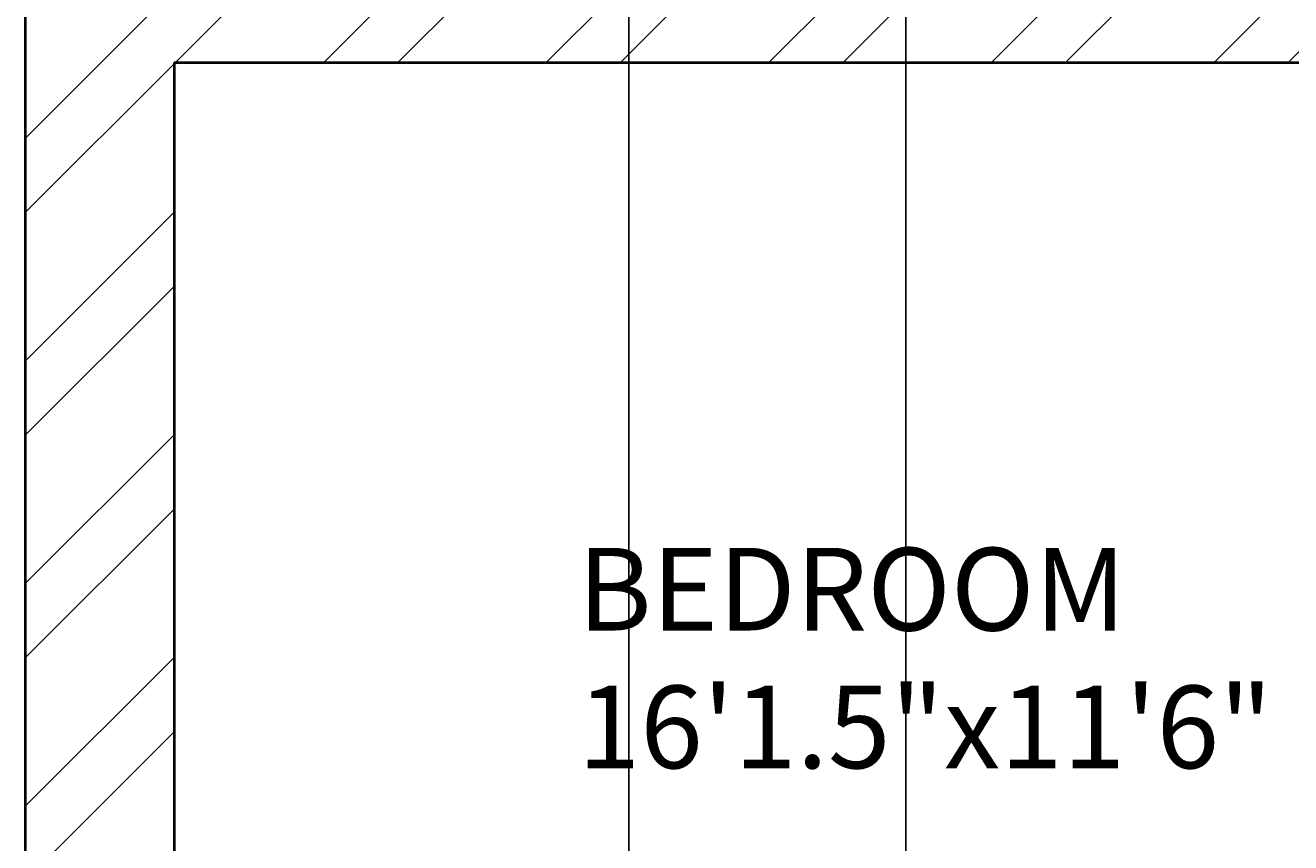
# Model space of a CAD drawing. Units: inches. Extents: x 1601 to 2297, y 1496 to 2631.
# Tile 34 of 57: x 1686 to 1763, y 2236 to 2286. Entities that reach past the tile are written whole.
import ezdxf

# ---------------------------------------------------------------- set-up
doc = ezdxf.new("R2010")
doc.units = ezdxf.units.IN
for name, color, linetype, lineweight in [('A-ANNO-DIMS', 2, 'Continuous', 18), ('A-AREA-IDEN', 7, 'Continuous', 18), ('A-WALL', 7, 'Continuous', 40), ('A-WALL-PATT', 215, 'Continuous', 13)]:
    doc.layers.add(name, color=color, linetype=linetype, lineweight=lineweight)
doc.styles.get("Standard").update_dxf_attribs({"font": 'arial.ttf'})
doc.dimstyles.get("Standard").update_dxf_attribs({"dimtxt": 0.18, "dimasz": 0.18, "dimexe": 0.18, "dimexo": 0.0625, "dimgap": 0.09, "dimtad": 0, "dimtih": 1, "dimtoh": 1, "dimdec": 4, "dimzin": 0, "dimdsep": 46, "dimtxsty": 'Standard', "dimcen": 0.09, "dimadec": 0, "dimazin": 0, "dimtfac": 1, "dimtdec": 4, "dimtofl": 0, "dimtmove": 0, "dimatfit": 3, "dimfxl": 1, "dimtolj": 1, "dimtzin": 0, "dimarcsym": 0})

# ---------------------------------------------------------------- blocks, each defined once
blk = doc.blocks.new('*D32')
at = {"layer": 'A-ANNO-DIMS', "color": 0, "lineweight": -2, "transparency": 16777216}
for p, q in [((1686.037, 2031.388), (1686.037, 2581.055)), ((1686.217, 2580.875), (1703.909, 2580.875)), ((1722.389, 2580.875), (1704.697, 2580.875)), ((1722.569, 2031.388), (1722.569, 2581.055))]:
    blk.add_line(p, q, dxfattribs=at)
at = {"layer": 'A-ANNO-DIMS', "color": 0, "transparency": 16777216}
for points in [[(1686.217, 2580.905), (1686.217, 2580.845), (1686.037, 2580.875)], [(1722.389, 2580.905), (1722.389, 2580.845), (1722.569, 2580.875)]]:
    blk.add_solid(points, dxfattribs=at)
at = {"layer": 'Defpoints', "color": 0, "transparency": 16777216}
for p in [(1722.569, 2580.875), (1686.037, 2031.325), (1722.569, 2031.325)]:
    blk.add_point(p, dxfattribs=at)
at = {"layer": 'A-ANNO-DIMS', "color": 0, "transparency": 16777216, "insert": (1704.303, 2580.875), "char_height": 0.18, "attachment_point": 5}
blk.add_mtext('\\A1;36.53', dxfattribs=at)
blk = doc.blocks.new('*D36')
at = {"layer": 'A-ANNO-DIMS', "color": 0, "lineweight": -2, "transparency": 16777216}
for p, q in [((1686.037, 1635.388), (1686.037, 2581.055)), ((1686.217, 2580.875), (1712.362, 2580.875)), ((1739.154, 2580.875), (1713.009, 2580.875)), ((1739.334, 1635.388), (1739.334, 2581.055))]:
    blk.add_line(p, q, dxfattribs=at)
at = {"layer": 'A-ANNO-DIMS', "color": 0, "transparency": 16777216}
for points in [[(1686.217, 2580.905), (1686.217, 2580.845), (1686.037, 2580.875)], [(1739.154, 2580.905), (1739.154, 2580.845), (1739.334, 2580.875)]]:
    blk.add_solid(points, dxfattribs=at)
at = {"layer": 'Defpoints', "color": 0, "transparency": 16777216}
for p in [(1739.334, 2580.875), (1686.037, 1635.325), (1739.334, 1635.325)]:
    blk.add_point(p, dxfattribs=at)
at = {"layer": 'A-ANNO-DIMS', "color": 0, "transparency": 16777216, "insert": (1712.685, 2580.875), "char_height": 0.18, "attachment_point": 5}
blk.add_mtext('\\A1;53.3', dxfattribs=at)

msp = doc.modelspace()

# ---------------------------------------------------------------- hatches: boundary and pattern name
at = {"layer": 'A-WALL-PATT'}
h = msp.add_hatch(dxfattribs=at)
h.set_pattern_fill('ANSI32', color=256)
h.paths.add_polyline_path([(1842.0336, 2528.0767), (1842.0336, 2532.3254), (1686.0373, 2532.3254), (1686.0373, 2492.9493), (1695.0373, 2492.9493), (1695.0373, 2523.3254), (1827.0373, 2523.3254), (1827.0373, 2416.8254), (1834.6225, 2416.8254), (1834.6225, 2419.0754), (1834.6225, 2421.3254), (1831.5373, 2421.3254), (1831.5373, 2523.3254), (1842.0336, 2523.3254)])
h.paths.add_polyline_path([(1695.0373, 2432.9493), (1686.0373, 2432.9493), (1686.0373, 2325.989), (1695.0373, 2325.989), (1695.0373, 2347.8254), (1827.0373, 2347.8254), (1827.0373, 2287.8254), (1823.2991, 2287.8254), (1823.2991, 2283.3254), (1847.9422, 2283.3254), (1847.9422, 2285.5754), (1847.9422, 2287.8254), (1831.5373, 2287.8254), (1831.5373, 2347.8254), (1846.9946, 2347.8254), (1846.9946, 2350.0754), (1846.9946, 2352.3254), (1695.0373, 2352.3254)])
h.paths.add_polyline_path([(1807.1169, 1573.5395), (2055.0405, 1573.5395), (2055.0405, 1610.6322), (1807.1169, 1610.6322)], flags=9)
h.paths.add_polyline_path([(1841.1631, 1712.7967), (1870.3957, 1712.7967), (1870.3957, 1731.454), (1841.1631, 1731.454)], flags=9)
h.paths.add_polyline_path([(2144.3862, 1772.185), (2191.0233, 1772.185), (2191.0233, 1790.8423), (2144.3862, 1790.8423)], flags=9)
h.paths.add_polyline_path([(2143.0128, 1827.3312), (2177.9958, 1827.3312), (2177.9958, 1845.9886), (2143.0128, 1845.9886)], flags=9)
h.paths.add_polyline_path([(2041.2439, 1833.5691), (2070.8516, 1833.5691), (2070.8516, 1852.2264), (2041.2439, 1852.2264)], flags=9)
h.paths.add_polyline_path([(2097.2791, 1947.0598), (2134.2061, 1947.0598), (2134.2061, 1965.7171), (2097.2791, 1965.7171)], flags=9)
h.paths.add_polyline_path([(2214.995, 1904.3124), (2214.995, 1942.2899), (2196.3376, 1942.2899), (2196.3376, 1904.3124)], flags=9)
h.paths.add_polyline_path([(2186.6284, 2043.8031), (2219.7935, 2043.8031), (2219.7935, 2062.4605), (2186.6284, 2062.4605)], flags=9)
h.paths.add_polyline_path([(2064.0877, 2031.616), (2097.4949, 2031.616), (2097.4949, 2050.2734), (2064.0877, 2050.2734)], flags=9)
h.paths.add_polyline_path([(1973.1349, 1986.0688), (2008.4009, 1986.0688), (2008.4009, 2004.7261), (1973.1349, 2004.7261)], flags=9)
h.paths.add_polyline_path([(1976.3676, 2106.9635), (2005.7469, 2106.9635), (2005.7469, 2125.6209), (1976.3676, 2125.6209)], flags=9)
h.paths.add_polyline_path([(1991.7852, 2180.4863), (2027.0513, 2180.4863), (2027.0513, 2199.1437), (1991.7852, 2199.1437)], flags=9)
h.paths.add_polyline_path([(2106.1801, 2187.9359), (2152.2101, 2187.9359), (2152.2101, 2206.5932), (2106.1801, 2206.5932)], flags=9)
h.paths.add_polyline_path([(2148.6686, 2262.2542), (2182.318, 2262.2542), (2182.318, 2280.9115), (2148.6686, 2280.9115)], flags=9)
h.paths.add_polyline_path([(2041.6327, 2252.8147), (2071.2405, 2252.8147), (2071.2405, 2271.4721), (2041.6327, 2271.4721)], flags=9)
h.paths.add_polyline_path([(2063.9734, 2375.4265), (2100.9004, 2375.4265), (2100.9004, 2394.0839), (2063.9734, 2394.0839)], flags=9)
h.paths.add_polyline_path([(2216.4955, 2330.9748), (2216.4955, 2370.2654), (2197.8381, 2370.2654), (2197.8381, 2330.9748)], flags=9)
h.paths.add_polyline_path([(2179.1416, 2485.8687), (2212.3067, 2485.8687), (2212.3067, 2504.5261), (2179.1416, 2504.5261)], flags=9)
h.paths.add_polyline_path([(2078.7442, 2471.1516), (2112.1514, 2471.1516), (2112.1514, 2489.809), (2078.7442, 2489.809)], flags=9)
h.paths.add_polyline_path([(1915.9631, 2329.4668), (1952.8902, 2329.4668), (1952.8902, 2348.1241), (1915.9631, 2348.1241)], flags=9)
h.paths.add_polyline_path([(1904.3189, 2499.6709), (1940.4512, 2499.6709), (1940.4512, 2518.3282), (1904.3189, 2518.3282)], flags=9)
h.paths.add_polyline_path([(1892.3665, 2100.4595), (1925.6374, 2100.4595), (1925.6374, 2119.1169), (1892.3665, 2119.1169)], flags=9)
h.paths.add_polyline_path([(1909.2984, 1805.9631), (1946.2254, 1805.9631), (1946.2254, 1824.6205), (1909.2984, 1824.6205)], flags=9)
h.paths.add_polyline_path([(1934.6056, 1658.616), (1970.738, 1658.616), (1970.738, 1677.2733), (1934.6056, 1677.2733)], flags=9)
h.paths.add_polyline_path([(1711.2052, 1789.8902), (1750.0456, 1789.8902), (1750.0456, 1808.5476), (1711.2052, 1808.5476)], flags=9)
h.paths.add_polyline_path([(1742.7874, 1854.6743), (1771.9449, 1854.6743), (1771.9449, 1873.3317), (1742.7874, 1873.3317)], flags=9)
h.paths.add_polyline_path([(1807.3592, 1997.7912), (1850.1116, 1997.7912), (1850.1116, 2016.4486), (1807.3592, 2016.4486)], flags=9)
h.paths.add_polyline_path([(1717.4579, 2237.7844), (1760.2103, 2237.7844), (1760.2103, 2256.4417), (1717.4579, 2256.4417)], flags=9)
h.paths.add_polyline_path([(1780.9285, 2324.0623), (1810.086, 2324.0623), (1810.086, 2342.7197), (1780.9285, 2342.7197)], flags=25)
h.paths.add_polyline_path([(1837.696, 2449.2024), (1866.9286, 2449.2024), (1866.9286, 2467.8598), (1837.696, 2467.8598)], flags=9)
h.paths.add_polyline_path([(1712.7752, 2484.9404), (1751.6156, 2484.9404), (1751.6156, 2503.5977), (1712.7752, 2503.5977)], flags=25)
h = msp.add_hatch(dxfattribs=at)
h.set_pattern_fill('ANSI32', color=256)
h.paths.add_polyline_path([(1973.9371, 2211.3254), (1893.0373, 2211.3254), (1893.0373, 2287.8254), (1884.6167, 2287.8254), (1884.6167, 2285.5754), (1884.6167, 2283.3254), (1888.5373, 2283.3254), (1888.5373, 2145.3254), (1695.0373, 2145.3254), (1695.0373, 2173.8724), (1690.5373, 2173.8724), (1686.0373, 2173.8724), (1686.0373, 2136.3254), (1722.5687, 2136.3254), (1722.5687, 2117.4352), (1731.5687, 2117.4352), (1731.5687, 2136.3254), (1893.0373, 2136.3254), (1893.0373, 2202.3254), (1959.0373, 2202.3254), (1959.0373, 2182.1303), (1968.0373, 2182.1303), (1968.0373, 2202.3254), (1973.9371, 2202.3254)])
h.paths.add_polyline_path([(2094.0373, 2274.6364), (2096.4294, 2274.6364), (2096.4294, 2276.8864), (2096.4294, 2279.1364), (2094.0373, 2279.1364), (2094.0373, 2290.8254), (2094.0373, 2295.3254), (2089.5373, 2295.3254), (2089.5373, 2230.8254), (2035.5373, 2230.8254), (2035.5373, 2299.8254), (2031.0373, 2299.8254), (2031.0373, 2211.3254), (2023.0065, 2211.3254), (2023.0065, 2202.3254), (2031.0373, 2202.3254), (2031.0373, 2140.8254), (1968.0373, 2140.8254), (1968.0373, 2145.9106), (1963.5373, 2145.9106), (1959.0373, 2145.9106), (1959.0373, 2116.839), (1963.5373, 2116.839), (1968.0373, 2116.839), (1968.0373, 2131.8254), (2031.0373, 2131.8254), (2031.0373, 2094.3254), (2031.0373, 2085.3254), (2031.0373, 2056.8254), (1968.0373, 2056.8254), (1968.0373, 2070.4947), (1963.5373, 2070.4947), (1959.0373, 2070.4947), (1959.0373, 2040.3029), (1968.0373, 2040.3029), (1968.0373, 2047.8254), (2031.0373, 2047.8254), (2031.0373, 1983.3254), (2031.0373, 1978.8254), (2021.1979, 1978.8254), (2021.1979, 1974.3254), (2031.0373, 1974.3254), (2031.0373, 1954.3528), (2035.5373, 1954.3528), (2035.5373, 1974.3254), (2035.5373, 1981.8254), (2055.5513, 1981.8254), (2055.5513, 1986.3254), (2035.5373, 1986.3254), (2035.5373, 2047.8254), (2040.0373, 2047.8254), (2040.0373, 2085.3254), (2040.0373, 2094.3254), (2040.0373, 2140.8254), (2035.5373, 2140.8254), (2035.5373, 2226.3254), (2089.5373, 2226.3254), (2094.0373, 2226.3254)])
h.paths.add_polyline_path([(2226.0373, 2230.8254), (2134.5373, 2230.8254), (2134.5373, 2233.5437), (2130.0373, 2233.5437), (2130.0373, 2226.3254), (2134.5373, 2226.3254), (2226.0373, 2226.3254)])
h.paths.add_polyline_path([(1807.1169, 1573.5395), (2055.0405, 1573.5395), (2055.0405, 1610.6322), (1807.1169, 1610.6322)], flags=9)
h.paths.add_polyline_path([(1841.1631, 1712.7967), (1870.3957, 1712.7967), (1870.3957, 1731.454), (1841.1631, 1731.454)], flags=9)
h.paths.add_polyline_path([(2144.3862, 1772.185), (2191.0233, 1772.185), (2191.0233, 1790.8423), (2144.3862, 1790.8423)], flags=9)
h.paths.add_polyline_path([(2143.0128, 1827.3312), (2177.9958, 1827.3312), (2177.9958, 1845.9886), (2143.0128, 1845.9886)], flags=9)
h.paths.add_polyline_path([(2041.2439, 1833.5691), (2070.8516, 1833.5691), (2070.8516, 1852.2264), (2041.2439, 1852.2264)], flags=9)
h.paths.add_polyline_path([(2097.2791, 1947.0598), (2134.2061, 1947.0598), (2134.2061, 1965.7171), (2097.2791, 1965.7171)], flags=9)
h.paths.add_polyline_path([(2214.995, 1904.3124), (2214.995, 1942.2899), (2196.3376, 1942.2899), (2196.3376, 1904.3124)], flags=9)
h.paths.add_polyline_path([(2186.6284, 2043.8031), (2219.7935, 2043.8031), (2219.7935, 2062.4605), (2186.6284, 2062.4605)], flags=9)
h.paths.add_polyline_path([(2064.0877, 2031.616), (2097.4949, 2031.616), (2097.4949, 2050.2734), (2064.0877, 2050.2734)], flags=9)
h.paths.add_polyline_path([(1973.1349, 1986.0688), (2008.4009, 1986.0688), (2008.4009, 2004.7261), (1973.1349, 2004.7261)], flags=25)
h.paths.add_polyline_path([(1976.3676, 2106.9635), (2005.7469, 2106.9635), (2005.7469, 2125.6209), (1976.3676, 2125.6209)], flags=25)
h.paths.add_polyline_path([(1991.7852, 2180.4863), (2027.0513, 2180.4863), (2027.0513, 2199.1437), (1991.7852, 2199.1437)], flags=25)
h.paths.add_polyline_path([(2106.1801, 2187.9359), (2152.2101, 2187.9359), (2152.2101, 2206.5932), (2106.1801, 2206.5932)], flags=9)
h.paths.add_polyline_path([(2148.6686, 2262.2542), (2182.318, 2262.2542), (2182.318, 2280.9115), (2148.6686, 2280.9115)], flags=9)
h.paths.add_polyline_path([(2041.6327, 2252.8147), (2071.2405, 2252.8147), (2071.2405, 2271.4721), (2041.6327, 2271.4721)], flags=25)
h.paths.add_polyline_path([(2063.9734, 2375.4265), (2100.9004, 2375.4265), (2100.9004, 2394.0839), (2063.9734, 2394.0839)], flags=9)
h.paths.add_polyline_path([(2216.4955, 2330.9748), (2216.4955, 2370.2654), (2197.8381, 2370.2654), (2197.8381, 2330.9748)], flags=9)
h.paths.add_polyline_path([(2179.1416, 2485.8687), (2212.3067, 2485.8687), (2212.3067, 2504.5261), (2179.1416, 2504.5261)], flags=9)
h.paths.add_polyline_path([(2078.7442, 2471.1516), (2112.1514, 2471.1516), (2112.1514, 2489.809), (2078.7442, 2489.809)], flags=9)
h.paths.add_polyline_path([(1915.9631, 2329.4668), (1952.8902, 2329.4668), (1952.8902, 2348.1241), (1915.9631, 2348.1241)], flags=9)
h.paths.add_polyline_path([(1904.3189, 2499.6709), (1940.4512, 2499.6709), (1940.4512, 2518.3282), (1904.3189, 2518.3282)], flags=9)
h.paths.add_polyline_path([(1892.3665, 2100.4595), (1925.6374, 2100.4595), (1925.6374, 2119.1169), (1892.3665, 2119.1169)], flags=9)
h.paths.add_polyline_path([(1909.2984, 1805.9631), (1946.2254, 1805.9631), (1946.2254, 1824.6205), (1909.2984, 1824.6205)], flags=9)
h.paths.add_polyline_path([(1934.6056, 1658.616), (1970.738, 1658.616), (1970.738, 1677.2733), (1934.6056, 1677.2733)], flags=9)
h.paths.add_polyline_path([(1711.2052, 1789.8902), (1750.0456, 1789.8902), (1750.0456, 1808.5476), (1711.2052, 1808.5476)], flags=9)
h.paths.add_polyline_path([(1742.7874, 1854.6743), (1771.9449, 1854.6743), (1771.9449, 1873.3317), (1742.7874, 1873.3317)], flags=9)
h.paths.add_polyline_path([(1807.3592, 1997.7912), (1850.1116, 1997.7912), (1850.1116, 2016.4486), (1807.3592, 2016.4486)], flags=9)
h.paths.add_polyline_path([(1717.4579, 2237.7844), (1760.2103, 2237.7844), (1760.2103, 2256.4417), (1717.4579, 2256.4417)], flags=25)
h.paths.add_polyline_path([(1780.9285, 2324.0623), (1810.086, 2324.0623), (1810.086, 2342.7197), (1780.9285, 2342.7197)], flags=9)
h.paths.add_polyline_path([(1837.696, 2449.2024), (1866.9286, 2449.2024), (1866.9286, 2467.8598), (1837.696, 2467.8598)], flags=9)
h.paths.add_polyline_path([(1712.7752, 2484.9404), (1751.6156, 2484.9404), (1751.6156, 2503.5977), (1712.7752, 2503.5977)], flags=9)
h = msp.add_hatch(dxfattribs=at)
h.set_pattern_fill('ANSI32', color=256)
h.paths.add_polyline_path([(2230.5373, 1861.8254), (2182.5373, 1861.8254), (2182.5373, 1885.3637), (2178.0373, 1885.3637), (2178.0373, 1861.8254), (2166.0373, 1861.8254), (2134.5373, 1861.8254), (2130.0373, 1861.8254), (2130.0373, 1841.4682), (2126.8833, 1841.4682), (2126.8833, 1836.9682), (2130.0373, 1836.9682), (2130.0373, 1822.7302), (2134.5373, 1822.7302), (2134.5373, 1857.3254), (2166.0373, 1857.3254), (2226.0373, 1857.3254), (2226.0373, 1846.1155), (2230.5373, 1846.1155)])
h.paths.add_polyline_path([(2226.0373, 1797.3254), (2134.5373, 1797.3254), (2134.5373, 1800.6636), (2132.2873, 1800.6636), (2130.0373, 1800.6636), (2130.0373, 1797.3254), (2130.0373, 1792.8254), (2167.7264, 1792.8254), (2226.0373, 1792.8254)])
h.paths.add_polyline_path([(2230.5373, 1822.1155), (2226.0373, 1822.1155), (2226.0373, 1760.8563), (2230.5373, 1760.8563)])
h.paths.add_polyline_path([(2230.5373, 1700.8563), (2226.0373, 1700.8563), (2226.0373, 1644.3254), (2140.2517, 1644.3254), (2140.2517, 1635.3254), (2230.5373, 1635.3254)])
h.paths.add_polyline_path([(2080.2517, 1639.8254), (2080.2517, 1644.3254), (2035.5373, 1644.3254), (2035.5373, 1792.8254), (2094.0373, 1792.8254), (2094.0373, 1797.3254), (2094.0373, 1836.9682), (2097.1057, 1836.9682), (2097.1057, 1839.2182), (2097.1057, 1841.4682), (2094.0373, 1841.4682), (2094.0373, 1862.2276), (2089.5373, 1862.2276), (2089.5373, 1797.3254), (2035.5373, 1797.3254), (2035.5373, 1857.3254), (2035.5373, 1885.0916), (2031.0373, 1885.0916), (2031.0373, 1710.3254), (2012.329, 1710.3254), (2012.329, 1701.3254), (2031.0373, 1701.3254), (2031.0373, 1644.3254), (2031.0373, 1635.3254), (2080.2517, 1635.3254)])
h.paths.add_polyline_path([(1836.0373, 1653.2033), (1842.6171, 1653.2033), (1842.6171, 1657.7033), (1842.6171, 1662.2033), (1831.5373, 1662.2033), (1831.5373, 1764.2033), (1835.3881, 1764.2033), (1835.3881, 1766.4533), (1835.3881, 1768.7033), (1831.5373, 1768.7033), (1827.0373, 1768.7033), (1827.0373, 1662.2033), (1827.0373, 1635.3254), (1836.0373, 1635.3254)])
h.paths.add_polyline_path([(1893.0373, 1701.3254), (1907.193, 1701.3254), (1907.193, 1705.8254), (1907.193, 1710.3254), (1893.0373, 1710.3254), (1893.0373, 1819.8254), (1882.6444, 1819.8254), (1882.6444, 1817.5754), (1882.6444, 1815.3254), (1888.5373, 1815.3254), (1888.5373, 1662.2033), (1884.0373, 1662.2033), (1866.6171, 1662.2033), (1866.6171, 1653.2033), (1882.391, 1653.2033), (1884.0373, 1653.2033), (1884.0373, 1635.3254), (1893.0373, 1635.3254)])
h.paths.add_polyline_path([(1739.3335, 1639.8254), (1739.3335, 1644.3254), (1695.0373, 1644.3254), (1695.0373, 1702.0135), (1690.5373, 1702.0135), (1686.0373, 1702.0135), (1686.0373, 1635.3254), (1739.3335, 1635.3254)])
h.paths.add_polyline_path([(1827.0373, 1644.3254), (1799.3335, 1644.3254), (1799.3335, 1635.3254), (1827.0373, 1635.3254)])
h.paths.add_polyline_path([(1695.0373, 1815.3254), (1849.2759, 1815.3254), (1849.2759, 1819.8254), (1807.5373, 1819.8254), (1807.5373, 1879.8254), (1851.1533, 1879.8254), (1851.1533, 1882.0754), (1851.1533, 1884.3254), (1799.3405, 1884.3254), (1799.3405, 1882.0754), (1799.3405, 1879.8254), (1803.0373, 1879.8254), (1803.0373, 1819.8254), (1695.0373, 1819.8254), (1695.0373, 1835.0458), (1690.5373, 1835.0458), (1686.0373, 1835.0458), (1686.0373, 1766.1753), (1695.0373, 1766.1753)])
h.paths.add_polyline_path([(1775.8157, 1884.3254), (1695.0373, 1884.3254), (1695.0373, 1912.9526), (1690.5373, 1912.9526), (1686.0373, 1912.9526), (1686.0373, 1859.0458), (1695.0373, 1859.0458), (1695.0373, 1879.8254), (1775.8157, 1879.8254)])
h.paths.add_polyline_path([(1893.0373, 2031.3254), (1731.5687, 2031.3254), (1731.5687, 2057.4352), (1722.5687, 2057.4352), (1722.5687, 2031.3254), (1686.0373, 2031.3254), (1686.0373, 1972.9526), (1695.0373, 1972.9526), (1695.0373, 2022.3254), (1888.5373, 2022.3254), (1888.5373, 1884.3254), (1883.4996, 1884.3254), (1883.4996, 1879.8254), (1893.0373, 1879.8254), (1893.0373, 1974.3254), (1976.6199, 1974.3254), (1976.6199, 1978.8254), (1968.0373, 1978.8254), (1968.0373, 1983.3254), (1968.0373, 2008.4756), (1963.5373, 2008.4756), (1959.0373, 2008.4756), (1959.0373, 1983.3254), (1893.0373, 1983.3254)])
h.paths.add_polyline_path([(2230.5373, 2140.4745), (2226.0373, 2140.4745), (2226.0373, 2094.3254), (2040.0373, 2094.3254), (2040.0373, 2085.3254), (2178.0373, 2085.3254), (2178.0373, 2065.6965), (2182.5373, 2065.6965), (2182.5373, 2085.3254), (2226.0373, 2085.3254), (2226.0373, 1986.3254), (2211.2679, 1986.3254), (2211.2679, 1981.8254), (2230.5373, 1981.8254)])
h.paths.add_polyline_path([(2187.6292, 1986.3254), (2182.5373, 1986.3254), (2182.5373, 2029.6965), (2178.0373, 2029.6965), (2178.0373, 1986.3254), (2099.05, 1986.3254), (2099.05, 1981.8254), (2178.0373, 1981.8254), (2178.0373, 1969.3637), (2182.5373, 1969.3637), (2182.5373, 1981.8254), (2187.6292, 1981.8254), (2187.6292, 1984.0754)])
h.paths.add_polyline_path([(1807.1169, 1573.5395), (2055.0405, 1573.5395), (2055.0405, 1610.6322), (1807.1169, 1610.6322)], flags=9)
h.paths.add_polyline_path([(1841.1631, 1712.7967), (1870.3957, 1712.7967), (1870.3957, 1731.454), (1841.1631, 1731.454)], flags=9)
h.paths.add_polyline_path([(2144.3862, 1772.185), (2191.0233, 1772.185), (2191.0233, 1790.8423), (2144.3862, 1790.8423)], flags=9)
h.paths.add_polyline_path([(2143.0128, 1827.3312), (2177.9958, 1827.3312), (2177.9958, 1845.9886), (2143.0128, 1845.9886)], flags=25)
h.paths.add_polyline_path([(2041.2439, 1833.5691), (2070.8516, 1833.5691), (2070.8516, 1852.2264), (2041.2439, 1852.2264)], flags=25)
h.paths.add_polyline_path([(2097.2791, 1947.0598), (2134.2061, 1947.0598), (2134.2061, 1965.7171), (2097.2791, 1965.7171)], flags=9)
h.paths.add_polyline_path([(2214.995, 1904.3124), (2214.995, 1942.2899), (2196.3376, 1942.2899), (2196.3376, 1904.3124)], flags=9)
h.paths.add_polyline_path([(2186.6284, 2043.8031), (2219.7935, 2043.8031), (2219.7935, 2062.4605), (2186.6284, 2062.4605)], flags=25)
h.paths.add_polyline_path([(2064.0877, 2031.616), (2097.4949, 2031.616), (2097.4949, 2050.2734), (2064.0877, 2050.2734)], flags=25)
h.paths.add_polyline_path([(1973.1349, 1986.0688), (2008.4009, 1986.0688), (2008.4009, 2004.7261), (1973.1349, 2004.7261)], flags=9)
h.paths.add_polyline_path([(1976.3676, 2106.9635), (2005.7469, 2106.9635), (2005.7469, 2125.6209), (1976.3676, 2125.6209)], flags=9)
h.paths.add_polyline_path([(1991.7852, 2180.4863), (2027.0513, 2180.4863), (2027.0513, 2199.1437), (1991.7852, 2199.1437)], flags=9)
h.paths.add_polyline_path([(2106.1801, 2187.9359), (2152.2101, 2187.9359), (2152.2101, 2206.5932), (2106.1801, 2206.5932)], flags=9)
h.paths.add_polyline_path([(2148.6686, 2262.2542), (2182.318, 2262.2542), (2182.318, 2280.9115), (2148.6686, 2280.9115)], flags=9)
h.paths.add_polyline_path([(2041.6327, 2252.8147), (2071.2405, 2252.8147), (2071.2405, 2271.4721), (2041.6327, 2271.4721)], flags=9)
h.paths.add_polyline_path([(2063.9734, 2375.4265), (2100.9004, 2375.4265), (2100.9004, 2394.0839), (2063.9734, 2394.0839)], flags=9)
h.paths.add_polyline_path([(2216.4955, 2330.9748), (2216.4955, 2370.2654), (2197.8381, 2370.2654), (2197.8381, 2330.9748)], flags=9)
h.paths.add_polyline_path([(2179.1416, 2485.8687), (2212.3067, 2485.8687), (2212.3067, 2504.5261), (2179.1416, 2504.5261)], flags=9)
h.paths.add_polyline_path([(2078.7442, 2471.1516), (2112.1514, 2471.1516), (2112.1514, 2489.809), (2078.7442, 2489.809)], flags=9)
h.paths.add_polyline_path([(1915.9631, 2329.4668), (1952.8902, 2329.4668), (1952.8902, 2348.1241), (1915.9631, 2348.1241)], flags=9)
h.paths.add_polyline_path([(1904.3189, 2499.6709), (1940.4512, 2499.6709), (1940.4512, 2518.3282), (1904.3189, 2518.3282)], flags=9)
h.paths.add_polyline_path([(1892.3665, 2100.4595), (1925.6374, 2100.4595), (1925.6374, 2119.1169), (1892.3665, 2119.1169)], flags=9)
h.paths.add_polyline_path([(1909.2984, 1805.9631), (1946.2254, 1805.9631), (1946.2254, 1824.6205), (1909.2984, 1824.6205)], flags=9)
h.paths.add_polyline_path([(1934.6056, 1658.616), (1970.738, 1658.616), (1970.738, 1677.2733), (1934.6056, 1677.2733)], flags=9)
h.paths.add_polyline_path([(1711.2052, 1789.8902), (1750.0456, 1789.8902), (1750.0456, 1808.5476), (1711.2052, 1808.5476)], flags=25)
h.paths.add_polyline_path([(1742.7874, 1854.6743), (1771.9449, 1854.6743), (1771.9449, 1873.3317), (1742.7874, 1873.3317)], flags=25)
h.paths.add_polyline_path([(1807.3592, 1997.7912), (1850.1116, 1997.7912), (1850.1116, 2016.4486), (1807.3592, 2016.4486)], flags=25)
h.paths.add_polyline_path([(1717.4579, 2237.7844), (1760.2103, 2237.7844), (1760.2103, 2256.4417), (1717.4579, 2256.4417)], flags=9)
h.paths.add_polyline_path([(1780.9285, 2324.0623), (1810.086, 2324.0623), (1810.086, 2342.7197), (1780.9285, 2342.7197)], flags=9)
h.paths.add_polyline_path([(1837.696, 2449.2024), (1866.9286, 2449.2024), (1866.9286, 2467.8598), (1837.696, 2467.8598)], flags=9)
h.paths.add_polyline_path([(1712.7752, 2484.9404), (1751.6156, 2484.9404), (1751.6156, 2503.5977), (1712.7752, 2503.5977)], flags=9)
h = msp.add_hatch(dxfattribs=at)
h.set_pattern_fill('ANSI32', color=256)
h.paths.add_polyline_path([(1695.0373, 2283.3254), (1801.5627, 2283.3254), (1801.5627, 2285.5754), (1801.5627, 2287.8254), (1695.0373, 2287.8254), (1695.0373, 2301.989), (1690.5373, 2301.989), (1686.0373, 2301.989), (1686.0373, 2233.8724), (1695.0373, 2233.8724)])

# ---------------------------------------------------------------- linework, layer by layer
at = {"layer": 'A-WALL'}
for p, q in [((1686.0373, 2301.989), (1686.0373, 2233.8724)), ((1695.0373, 2283.3254), (1801.5627, 2283.3254)), ((1695.0373, 2283.3254), (1695.0373, 2233.8724))]:
    msp.add_line(p, q, dxfattribs=at)

# ---------------------------------------------------------------- texts
at = {"layer": 'A-AREA-IDEN', "insert": (1719.4684, 2253.9571), "char_height": 5, "attachment_point": 1}
msp.add_mtext_dynamic_manual_height_columns('BEDROOM\\P16\'1.5"x11\'6"', width=121.436148, gutter_width=12.5, heights=[0], dxfattribs=at)

# ---------------------------------------------------------------- dimensions: what is measured, and where the dimension line sits
at = {"layer": 'A-ANNO-DIMS'}
for base, p1, p2, override, picture, middle in [((1722.5687, 2580.8754), (1686.0373, 2031.3254), (1722.5687, 2031.3254), {"dimdec": 2, "dimlfac": 1, "dimrnd": 0, "dimzin": 0, "dimdsep": 46, "dimlunit": 2}, '*D32', (1704.303, 2580.8754)), ((1739.3335, 2580.8754), (1686.0373, 1635.3254), (1739.3335, 1635.3254), {"dimdec": 1, "dimlfac": 1, "dimrnd": 0, "dimzin": 0, "dimdsep": 46, "dimlunit": 2}, '*D36', (1712.6854, 2580.8754))]:
    dim = msp.add_linear_dim(base=base, p1=p1, p2=p2, dimstyle='Standard', override=override, dxfattribs=at)
    dim.commit()
    dim.dimension.update_dxf_attribs({"geometry": picture, "text_midpoint": middle})

doc.saveas('drawing.dxf')
